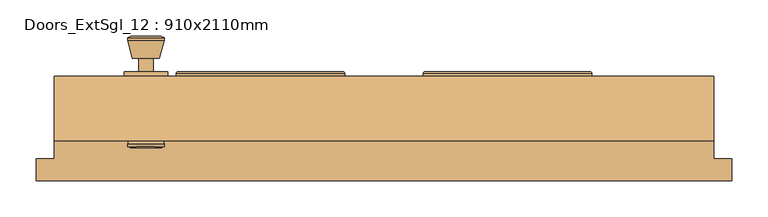
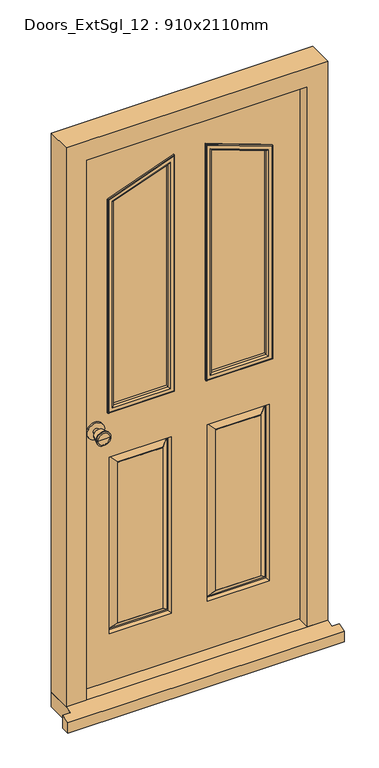
"""IFC4 building model written with IfcOpenShell, lengths in millimetres: door geometry, Doors_ExtSgl_12 : 910x2110mm."""

from ifc_helpers import new_model, si_unit, point, frame, frame_2d, origin, place, context, project, spatial, polyline, circle_curve, ellipse_curve, trimmed, segment, composite_curve, outline, extrude, faceted_brep, source, transform, mapped, element, save
from ifc_brep_helpers import plane_surface, cylinder_surface, revolved_surface, advanced_brep


def doors_extsgl_12_910x2110mm_ece77ece(model_context):
    return source(origin(), model_context, "Body", "SolidModel", [
        advanced_brep(
        [(-328.5, 18.4, 1000.0), (-338.5, 18.4, 1000.0), (-318.5, 18.4, 1000.0), (-308.0241324, 67.4, 1000.0), (-348.9758676, 67.4, 1000.0), (-328.5, 67.4, 1000.0), (-303.5, 65.5721319, 1000.0), (-353.5, 65.5721319, 1000.0), (-303.5, 62.1084537, 1000.0), (-353.5, 62.1084537, 1000.0), (-309.863764, 37.4, 1000.0), (-347.136236, 37.4, 1000.0), (-318.5, 37.4, 1000.0), (-338.5, 37.4, 1000.0)],
        [
            (0, 1),
            (1, 2, circle_curve(frame((-328.5, 18.4, 1000.0), z_axis=(0.0, -1.0, 0.0), x_axis=(-1.0, 0.0, 0.0)), 10.0)),
            (2, 0),
            (2, 1, circle_curve(frame((-328.5, 18.4, 1000.0), z_axis=(0.0, -1.0, 0.0), x_axis=(-1.0, 0.0, 0.0)), 10.0)),
            (3, 4, circle_curve(frame((-328.5, 67.4, 1000.0), z_axis=(0.0, 1.0, 0.0), x_axis=(-1.0, 0.0, 0.0)), 20.4758676)),
            (4, 5),
            (5, 3),
            (4, 3, circle_curve(frame((-328.5, 67.4, 1000.0), z_axis=(0.0, 1.0, 0.0), x_axis=(-1.0, 0.0, 0.0)), 20.4758676)),
            (6, 7, circle_curve(frame((-328.5, 65.5721319, 1000.0), z_axis=(0.0, 1.0, 0.0), x_axis=(-1.0, 0.0, 0.0)), 25.0)),
            (7, 4),
            (3, 6),
            (7, 6, circle_curve(frame((-328.5, 65.5721319, 1000.0), z_axis=(0.0, 1.0, 0.0), x_axis=(-1.0, 0.0, 0.0)), 25.0)),
            (8, 9, circle_curve(frame((-328.5, 62.1084537, 1000.0), z_axis=(0.0, 1.0, 0.0), x_axis=(-1.0, 0.0, 0.0)), 25.0)),
            (9, 7),
            (6, 8),
            (9, 8, circle_curve(frame((-328.5, 62.1084537, 1000.0), z_axis=(0.0, 1.0, 0.0), x_axis=(-1.0, 0.0, 0.0)), 25.0)),
            (10, 11, circle_curve(frame((-328.5, 37.4, 1000.0), z_axis=(0.0, 1.0, 0.0), x_axis=(-1.0, 0.0, 0.0)), 18.636236)),
            (11, 9),
            (8, 10),
            (11, 10, circle_curve(frame((-328.5, 37.4, 1000.0), z_axis=(0.0, 1.0, 0.0), x_axis=(-1.0, 0.0, 0.0)), 18.636236)),
            (12, 13, circle_curve(frame((-328.5, 37.4, 1000.0), z_axis=(0.0, 1.0, 0.0), x_axis=(-1.0, 0.0, 0.0)), 10.0)),
            (13, 11),
            (10, 12),
            (13, 12, circle_curve(frame((-328.5, 37.4, 1000.0), z_axis=(0.0, 1.0, 0.0), x_axis=(-1.0, 0.0, 0.0)), 10.0)),
            (1, 13),
            (12, 2),
        ],
        [
            plane_surface(frame((-328.5, 18.4, 1000.0), z_axis=(0.0, -1.0, 0.0), x_axis=(-1.0, 0.0, 0.0))),
            plane_surface(frame((-328.5, 67.4, 1000.0), z_axis=(0.0, 1.0, 0.0), x_axis=(-1.0, 0.0, 0.0))),
            revolved_surface(polyline([(-348.9758676, 67.4, 1000.0), (-353.5, 65.5721319, 1000.0)]), (-328.5, 18.4, 1000.0), (0.0, -1.0, 0.0)),
            cylinder_surface(frame((-328.5, 18.4, 1000.0), z_axis=(0.0, -1.0, 0.0), x_axis=(-1.0, 0.0, 0.0)), 25.0),
            revolved_surface(polyline([(-353.5, 62.1084537, 1000.0), (-347.136236, 37.4, 1000.0)]), (-328.5, 18.4, 1000.0), (0.0, -1.0, 0.0)),
            plane_surface(frame((-328.5, 37.4, 1000.0), z_axis=(0.0, -1.0, 0.0), x_axis=(-1.0, 0.0, 0.0))),
            cylinder_surface(frame((-328.5, 18.4, 1000.0), z_axis=(0.0, -1.0, 0.0), x_axis=(-1.0, 0.0, 0.0)), 10.0),
        ],
        [
            (0, [[1, 2, 3]]),
            (0, [[-3, 4, -1]]),
            (1, [[5, 6, 7]]),
            (1, [[8, -7, -6]]),
            (2, [[9, 10, -5, 11]]),
            (2, [[12, -11, -8, -10]]),
            (3, [[13, 14, -9, 15]]),
            (3, [[16, -15, -12, -14]]),
            (4, [[17, 18, -13, 19]]),
            (4, [[20, -19, -16, -18]]),
            (5, [[21, 22, -17, 23]]),
            (5, [[24, -23, -20, -22]]),
            (6, [[-2, 25, -21, 26]]),
            (6, [[-4, -26, -24, -25]]),
        ],
    ),
        extrude(outline(composite_curve([segment(trimmed(circle_curve(frame_2d((1000.0, -328.5)), 30.0), [point((1000.0, -358.5))], [point((1000.0, -298.5))], False, "CARTESIAN"), True, "CONTINUOUS"), segment(trimmed(circle_curve(frame_2d((1000.0, -328.5)), 30.0), [point((1000.0, -298.5))], [point((1000.0, -358.5))], False, "CARTESIAN"), True, "CONTINUOUS")], self_intersect=False)), frame((0.0, 12.4, 0.0), z_axis=(0.0, 1.0, 0.0), x_axis=(0.0, 0.0, 1.0)), (0.0, 0.0, 1.0), 6.0),
        advanced_brep(
        [(-328.5, -37.6, 1000.0), (-318.5, -37.6, 1000.0), (-338.5, -37.6, 1000.0), (-308.0241324, -86.6, 1000.0), (-328.5, -86.6, 1000.0), (-348.9758676, -86.6, 1000.0), (-303.5, -84.7721319, 1000.0), (-353.5, -84.7721319, 1000.0), (-303.5, -81.3084537, 1000.0), (-353.5, -81.3084537, 1000.0), (-309.863764, -56.6, 1000.0), (-347.136236, -56.6, 1000.0), (-318.5, -56.6, 1000.0), (-338.5, -56.6, 1000.0)],
        [
            (0, 1),
            (1, 2, circle_curve(frame((-328.5, -37.6, 1000.0), z_axis=(0.0, 1.0, 0.0), x_axis=(-1.0, 0.0, 0.0)), 10.0)),
            (2, 0),
            (2, 1, circle_curve(frame((-328.5, -37.6, 1000.0), z_axis=(0.0, 1.0, 0.0), x_axis=(-1.0, 0.0, 0.0)), 10.0)),
            (3, 4),
            (4, 5),
            (5, 3, circle_curve(frame((-328.5, -86.6, 1000.0), z_axis=(0.0, -1.0, 0.0), x_axis=(-1.0, 0.0, 0.0)), 20.4758676)),
            (3, 5, circle_curve(frame((-328.5, -86.6, 1000.0), z_axis=(0.0, -1.0, 0.0), x_axis=(-1.0, 0.0, 0.0)), 20.4758676)),
            (6, 3),
            (5, 7),
            (7, 6, circle_curve(frame((-328.5, -84.7721319, 1000.0), z_axis=(0.0, -1.0, 0.0), x_axis=(-1.0, 0.0, 0.0)), 25.0)),
            (6, 7, circle_curve(frame((-328.5, -84.7721319, 1000.0), z_axis=(0.0, -1.0, 0.0), x_axis=(-1.0, 0.0, 0.0)), 25.0)),
            (8, 6),
            (7, 9),
            (9, 8, circle_curve(frame((-328.5, -81.3084537, 1000.0), z_axis=(0.0, -1.0, 0.0), x_axis=(-1.0, 0.0, 0.0)), 25.0)),
            (8, 9, circle_curve(frame((-328.5, -81.3084537, 1000.0), z_axis=(0.0, -1.0, 0.0), x_axis=(-1.0, 0.0, 0.0)), 25.0)),
            (10, 8),
            (9, 11),
            (11, 10, circle_curve(frame((-328.5, -56.6, 1000.0), z_axis=(0.0, -1.0, 0.0), x_axis=(-1.0, 0.0, 0.0)), 18.636236)),
            (10, 11, circle_curve(frame((-328.5, -56.6, 1000.0), z_axis=(0.0, -1.0, 0.0), x_axis=(-1.0, 0.0, 0.0)), 18.636236)),
            (12, 10),
            (11, 13),
            (13, 12, circle_curve(frame((-328.5, -56.6, 1000.0), z_axis=(0.0, -1.0, 0.0), x_axis=(-1.0, 0.0, 0.0)), 10.0)),
            (12, 13, circle_curve(frame((-328.5, -56.6, 1000.0), z_axis=(0.0, -1.0, 0.0), x_axis=(-1.0, 0.0, 0.0)), 10.0)),
            (1, 12),
            (13, 2),
        ],
        [
            plane_surface(frame((-328.5, -37.6, 1000.0), z_axis=(0.0, 1.0, 0.0), x_axis=(-1.0, 0.0, 0.0))),
            plane_surface(frame((-328.5, -86.6, 1000.0), z_axis=(0.0, -1.0, 0.0), x_axis=(-1.0, 0.0, 0.0))),
            revolved_surface(polyline([(-348.9758676, -86.6, 1000.0), (-353.5, -84.7721319, 1000.0)]), (-328.5, -37.6, 1000.0), (0.0, 1.0, 0.0)),
            cylinder_surface(frame((-328.5, -37.6, 1000.0), z_axis=(0.0, 1.0, 0.0), x_axis=(-1.0, 0.0, 0.0)), 25.0),
            revolved_surface(polyline([(-353.5, -81.3084537, 1000.0), (-347.136236, -56.6, 1000.0)]), (-328.5, -37.6, 1000.0), (0.0, 1.0, 0.0)),
            plane_surface(frame((-328.5, -56.6, 1000.0), z_axis=(0.0, 1.0, 0.0), x_axis=(-1.0, 0.0, 0.0))),
            cylinder_surface(frame((-328.5, -37.6, 1000.0), z_axis=(0.0, 1.0, 0.0), x_axis=(-1.0, 0.0, 0.0)), 10.0),
        ],
        [
            (0, [[1, 2, 3]]),
            (0, [[-3, 4, -1]]),
            (1, [[5, 6, 7]]),
            (1, [[-6, -5, 8]]),
            (2, [[9, -7, 10, 11]]),
            (2, [[-10, -8, -9, 12]]),
            (3, [[13, -11, 14, 15]]),
            (3, [[-14, -12, -13, 16]]),
            (4, [[17, -15, 18, 19]]),
            (4, [[-18, -16, -17, 20]]),
            (5, [[21, -19, 22, 23]]),
            (5, [[-22, -20, -21, 24]]),
            (6, [[25, -23, 26, -2]]),
            (6, [[-26, -24, -25, -4]]),
        ],
    ),
        extrude(outline(composite_curve([segment(trimmed(circle_curve(frame_2d((1000.0, -328.5)), 30.0), [point((1000.0, -358.5))], [point((1000.0, -298.5))], False, "CARTESIAN"), True, "CONTINUOUS"), segment(trimmed(circle_curve(frame_2d((1000.0, -328.5)), 30.0), [point((1000.0, -298.5))], [point((1000.0, -358.5))], False, "CARTESIAN"), True, "CONTINUOUS")], self_intersect=False)), frame((0.0, -37.6, 0.0), z_axis=(0.0, 1.0, 0.0), x_axis=(0.0, 0.0, 1.0)), (0.0, 0.0, 1.0), 6.0),
        faceted_brep([(384.5, -76.6, 54.5), (384.5, -34.6, 54.5), (406.5, -34.6, 54.5), (406.5, 12.4, 54.5), (455.0, 12.4, 54.5), (455.0, -76.6, 54.5), (455.0, -76.6, 2110.0), (-455.0, -76.6, 2110.0), (-455.0, -76.6, 54.5), (-384.5, -76.6, 54.5), (-384.5, -76.6, 2039.5), (384.5, -76.6, 2039.5), (455.0, 12.4, 2110.0), (406.5, 12.4, 2061.5), (-406.5, 12.4, 2061.5), (-406.5, 12.4, 54.5), (-455.0, 12.4, 54.5), (-455.0, 12.4, 2110.0), (406.5, -34.6, 2061.5), (384.5, -34.6, 2039.5), (-384.5, -34.6, 2039.5), (-384.5, -34.6, 54.5), (-406.5, -34.6, 54.5), (-406.5, -34.6, 2061.5)], [[[0, 1, 2, 3, 4, 5]], [[5, 6, 7, 8, 9, 10, 11, 0]], [[4, 12, 6, 5]], [[3, 13, 14, 15, 16, 17, 12, 4]], [[2, 18, 13, 3]], [[1, 19, 20, 21, 22, 23, 18, 2]], [[0, 11, 19, 1]], [[9, 21, 20, 10]], [[8, 16, 15, 22, 21, 9]], [[7, 17, 16, 8]], [[14, 23, 22, 15]], [[6, 12, 17, 7]], [[13, 18, 23, 14]], [[10, 20, 19, 11]]]),
        faceted_brep([(403.5, 12.4, 58.5), (-404.4250294, 12.4, 58.5), (-404.4250294, 12.4, 2058.5), (403.5, 12.4, 2058.5), (62.5, 12.4, 1058.5), (278.5, 12.4, 1058.5), (278.5, 12.4, 1829.8824294), (62.5, 12.4, 1908.5), (-278.5, 12.4, 1058.5), (-62.5, 12.4, 1058.5), (-62.5, 12.4, 1908.5), (-278.5, 12.4, 1829.8824294), (-62.5, 12.4, 883.5), (-278.5, 12.4, 883.5), (-278.5, 12.4, 233.5), (-62.5, 12.4, 233.5), (278.5, 12.4, 883.5), (62.5, 12.4, 883.5), (62.5, 12.4, 233.5), (278.5, 12.4, 233.5), (-92.5, 12.4, 263.5), (-248.5, 12.4, 263.5), (-248.5, 12.4, 853.5), (-92.5, 12.4, 853.5), (248.5, 12.4, 263.5), (92.5, 12.4, 263.5), (92.5, 12.4, 853.5), (248.5, 12.4, 853.5), (403.5, -31.6, 58.5), (403.5, -31.6, 2058.5), (-404.4250294, -31.6, 2058.5), (-404.4250294, -31.6, 58.5), (62.5, -31.6, 1058.5), (62.5, -31.6, 1908.5), (278.5, -31.6, 1829.8824294), (278.5, -31.6, 1058.5), (-278.5, -31.6, 1058.5), (-278.5, -31.6, 1829.8824294), (-62.5, -31.6, 1908.5), (-62.5, -31.6, 1058.5), (62.5, -31.6, 883.5), (278.5, -31.6, 883.5), (278.5, -31.6, 233.5), (62.5, -31.6, 233.5), (-278.5, -31.6, 883.5), (-62.5, -31.6, 883.5), (-62.5, -31.6, 233.5), (-278.5, -31.6, 233.5), (92.5, -31.6, 263.5), (248.5, -31.6, 263.5), (248.5, -31.6, 853.5), (92.5, -31.6, 853.5), (-248.5, -31.6, 263.5), (-92.5, -31.6, 263.5), (-92.5, -31.6, 853.5), (-248.5, -31.6, 853.5), (65.5, -16.6, 880.5), (65.5, -16.6, 236.5), (90.5, -30.6, 855.5), (70.5, -16.6, 875.5), (70.5, -16.6, 241.5), (90.5, -30.6, 261.5), (92.5, -30.6, 853.5), (92.5, -30.6, 263.5), (275.5, -16.6, 236.5), (270.5, -16.6, 241.5), (250.5, -30.6, 261.5), (248.5, -30.6, 263.5), (275.5, -16.6, 880.5), (270.5, -16.6, 875.5), (250.5, -30.6, 855.5), (248.5, -30.6, 853.5), (-275.5, -16.6, 880.5), (-275.5, -16.6, 236.5), (-250.5, -30.6, 855.5), (-270.5, -16.6, 875.5), (-270.5, -16.6, 241.5), (-250.5, -30.6, 261.5), (-248.5, -30.6, 853.5), (-248.5, -30.6, 263.5), (-65.5, -16.6, 236.5), (-70.5, -16.6, 241.5), (-90.5, -30.6, 261.5), (-92.5, -30.6, 263.5), (-65.5, -16.6, 880.5), (-70.5, -16.6, 875.5), (-90.5, -30.6, 855.5), (-92.5, -30.6, 853.5), (-92.5, 11.4, 263.5), (-92.5, 11.4, 853.5), (-70.5, -2.6, 241.5), (-90.5, 11.4, 261.5), (-90.5, 11.4, 855.5), (-70.5, -2.6, 875.5), (-65.5, -2.6, 236.5), (-65.5, -2.6, 880.5), (-248.5, 11.4, 853.5), (-250.5, 11.4, 855.5), (-270.5, -2.6, 875.5), (-275.5, -2.6, 880.5), (-248.5, 11.4, 263.5), (-250.5, 11.4, 261.5), (-270.5, -2.6, 241.5), (-275.5, -2.6, 236.5), (275.5, -2.6, 880.5), (275.5, -2.6, 236.5), (250.5, 11.4, 855.5), (270.5, -2.6, 875.5), (270.5, -2.6, 241.5), (250.5, 11.4, 261.5), (248.5, 11.4, 853.5), (248.5, 11.4, 263.5), (65.5, -2.6, 236.5), (70.5, -2.6, 241.5), (90.5, 11.4, 261.5), (92.5, 11.4, 263.5), (65.5, -2.6, 880.5), (70.5, -2.6, 875.5), (90.5, 11.4, 855.5), (92.5, 11.4, 853.5)], [[[0, 1, 2, 3], [4, 5, 6, 7], [8, 9, 10, 11], [12, 13, 14, 15], [16, 17, 18, 19]], [[20, 21, 22, 23]], [[24, 25, 26, 27]], [[28, 29, 30, 31], [32, 33, 34, 35], [36, 37, 38, 39], [40, 41, 42, 43], [44, 45, 46, 47]], [[48, 49, 50, 51]], [[52, 53, 54, 55]], [[3, 29, 28, 0]], [[2, 30, 29, 3]], [[1, 31, 30, 2]], [[0, 28, 31, 1]], [[7, 33, 32, 4]], [[6, 34, 33, 7]], [[5, 35, 34, 6]], [[4, 32, 35, 5]], [[11, 37, 36, 8]], [[10, 38, 37, 11]], [[9, 39, 38, 10]], [[8, 36, 39, 9]], [[56, 40, 43, 57]], [[58, 59, 60, 61]], [[48, 51, 62, 63]], [[43, 42, 64, 57]], [[60, 65, 66, 61]], [[63, 67, 49, 48]], [[42, 41, 68, 64]], [[65, 69, 70, 66]], [[67, 71, 50, 49]], [[56, 68, 41, 40]], [[57, 64, 68, 56], [59, 69, 65, 60]], [[58, 70, 69, 59]], [[61, 66, 70, 58], [62, 71, 67, 63]], [[51, 50, 71, 62]], [[72, 44, 47, 73]], [[74, 75, 76, 77]], [[52, 55, 78, 79]], [[47, 46, 80, 73]], [[76, 81, 82, 77]], [[79, 83, 53, 52]], [[46, 45, 84, 80]], [[81, 85, 86, 82]], [[83, 87, 54, 53]], [[72, 84, 45, 44]], [[73, 80, 84, 72], [75, 85, 81, 76]], [[74, 86, 85, 75]], [[77, 82, 86, 74], [78, 87, 83, 79]], [[55, 54, 87, 78]], [[88, 20, 23, 89]], [[90, 91, 92, 93]], [[12, 15, 94, 95]], [[23, 22, 96, 89]], [[92, 97, 98, 93]], [[95, 99, 13, 12]], [[22, 21, 100, 96]], [[97, 101, 102, 98]], [[99, 103, 14, 13]], [[88, 100, 21, 20]], [[91, 101, 97, 92], [89, 96, 100, 88]], [[90, 102, 101, 91]], [[94, 103, 99, 95], [93, 98, 102, 90]], [[15, 14, 103, 94]], [[104, 16, 19, 105]], [[106, 107, 108, 109]], [[24, 27, 110, 111]], [[19, 18, 112, 105]], [[108, 113, 114, 109]], [[111, 115, 25, 24]], [[18, 17, 116, 112]], [[113, 117, 118, 114]], [[115, 119, 26, 25]], [[104, 116, 17, 16]], [[105, 112, 116, 104], [107, 117, 113, 108]], [[106, 118, 117, 107]], [[109, 114, 118, 106], [110, 119, 115, 111]], [[27, 26, 119, 110]]]),
        faceted_brep([(480.0, -131.6, 0.0), (480.0, -101.6, 0.0), (480.0, -101.6, 47.2703282), (480.0, -131.6, 38.5947221), (-480.0, -131.6, 38.5947221), (-480.0, -101.6, 47.2703282), (-480.0, -101.6, 0.0), (-480.0, -131.6, 0.0), (-455.0, -101.6, 0.0), (-455.0, 12.4, 0.0), (455.0, 12.4, 0.0), (455.0, -101.6, 0.0), (455.0, -101.6, 47.2703282), (455.0, -76.6, 54.5), (-455.0, -76.6, 54.5), (-455.0, -101.6, 47.2703282), (455.0, 12.4, 54.5), (-455.0, 12.4, 54.5)], [[[0, 1, 2, 3]], [[4, 5, 6, 7]], [[7, 6, 8, 9, 10, 11, 1, 0]], [[3, 4, 7, 0]], [[3, 2, 12, 13, 14, 15, 5, 4]], [[14, 13, 16, 17]], [[17, 16, 10, 9]], [[15, 14, 17, 9, 8]], [[8, 6, 5, 15]], [[11, 10, 16, 13, 12]], [[12, 2, 1, 11]]]),
        extrude(outline(polyline([(1058.5, 278.5), (1829.8824294, 278.5), (1908.5, 62.5), (1058.5, 62.5), (1058.5, 278.5)])), frame((0.0, -21.6, 0.0), z_axis=(0.0, 1.0, 0.0), x_axis=(0.0, 0.0, 1.0)), (0.0, 0.0, 1.0), 24.0),
        extrude(outline(polyline([(1058.5, -62.5), (1908.5, -62.5), (1829.8824294, -278.5), (1058.5, -278.5), (1058.5, -62.5)])), frame((0.0, -21.6, 0.0), z_axis=(0.0, 1.0, 0.0), x_axis=(0.0, 0.0, 1.0)), (0.0, 0.0, 1.0), 24.0),
        advanced_brep(
        [(286.5, -35.6, 1835.4840897), (286.5, -35.6, 1050.5), (286.5, -31.6, 1050.5), (286.5, -31.6, 1835.4840897), (284.5, -37.6, 1834.0836746), (284.5, -37.6, 1052.5), (266.5, -32.6, 1821.4799389), (266.5, -32.6, 1070.5), (271.5, -37.6, 1065.5), (271.5, -37.6, 1824.9809766), (266.5, -21.6, 1821.4799389), (266.5, -21.6, 1070.5), (278.5, -31.6, 1829.8824294), (278.5, -31.6, 1058.5), (278.5, -21.6, 1058.5), (278.5, -21.6, 1829.8824294), (54.5, -35.6, 1050.5), (54.5, -31.6, 1050.5), (56.5, -37.6, 1052.5), (74.5, -32.6, 1070.5), (69.5, -37.6, 1065.5), (74.5, -21.6, 1070.5), (62.5, -31.6, 1058.5), (62.5, -21.6, 1058.5), (54.5, -35.6, 1919.9251841), (54.5, -31.6, 1919.9251841), (56.5, -37.6, 1917.068888), (74.5, -32.6, 1891.3622239), (69.5, -37.6, 1898.502964), (74.5, -21.6, 1891.3622239), (62.5, -31.6, 1908.5), (62.5, -21.6, 1908.5)],
        [
            (0, 1),
            (1, 2),
            (2, 3),
            (3, 0),
            (4, 5),
            (5, 1, ellipse_curve(frame((284.5, -35.6, 1052.5), z_axis=(0.7071067811865475, 0.0, 0.7071067811865475), x_axis=(-0.7071067811865474, 0.0, 0.7071067811865476)), 2.8284271, 2.0)),
            (0, 4, ellipse_curve(frame((284.5, -35.6, 1834.0836746), z_axis=(0.5735764363510463, 0.0, -0.8191520442889918), x_axis=(0.8191520442889918, 0.0, 0.5735764363510459)), 2.4415492, 2.0)),
            (6, 7),
            (7, 8, ellipse_curve(frame((271.5, -32.6, 1065.5), z_axis=(0.7071067811865475, 0.0, 0.7071067811865475), x_axis=(-0.7071067811865474, 0.0, 0.7071067811865476)), 7.0710678, 5.0)),
            (8, 9),
            (9, 6, ellipse_curve(frame((271.5, -32.6, 1824.9809766), z_axis=(0.5735764363510463, 0.0, -0.8191520442889918), x_axis=(0.8191520442889918, 0.0, 0.5735764363510459)), 6.1038729, 5.0)),
            (10, 11),
            (11, 7),
            (6, 10),
            (12, 13),
            (13, 14),
            (14, 15),
            (15, 12),
            (1, 16),
            (16, 17),
            (17, 2),
            (5, 18),
            (18, 16, ellipse_curve(frame((56.5, -35.6, 1052.5), z_axis=(0.7071067811865475, 0.0, -0.7071067811865475), x_axis=(0.7071067811865476, 0.0, 0.7071067811865474)), 2.8284271, 2.0)),
            (7, 19),
            (19, 20, ellipse_curve(frame((69.5, -32.6, 1065.5), z_axis=(0.7071067811865475, 0.0, -0.7071067811865475), x_axis=(0.7071067811865476, 0.0, 0.7071067811865474)), 7.0710678, 5.0)),
            (20, 8),
            (11, 21),
            (21, 19),
            (13, 22),
            (22, 23),
            (23, 14),
            (16, 24),
            (24, 25),
            (25, 17),
            (18, 26),
            (26, 24, ellipse_curve(frame((56.5, -35.6, 1917.068888), z_axis=(-0.8191520442889917, 0.0, -0.5735764363510462), x_axis=(0.5735764363510462, 0.0, -0.8191520442889918)), 3.4868936, 2.0)),
            (19, 27),
            (27, 28, ellipse_curve(frame((69.5, -32.6, 1898.502964), z_axis=(-0.8191520442889917, 0.0, -0.5735764363510462), x_axis=(0.5735764363510462, 0.0, -0.8191520442889918)), 8.717234, 5.0)),
            (28, 20),
            (21, 29),
            (29, 27),
            (22, 30),
            (30, 31),
            (31, 23),
            (24, 0),
            (3, 25),
            (26, 4),
            (28, 9),
            (27, 6),
            (29, 10),
            (31, 15),
            (30, 12),
        ],
        [
            plane_surface(frame((286.5, -31.6, 1835.4840897), z_axis=(1.0, 0.0, 0.0), x_axis=(0.0, 0.0, -1.0))),
            cylinder_surface(frame((284.5, -35.6, 1829.8824294), z_axis=(0.0, 0.0, 1.0), x_axis=(1.0, 0.0, 0.0)), 2.0),
            cylinder_surface(frame((271.5, -32.6, 1829.8824294), z_axis=(0.0, 0.0, 1.0), x_axis=(1.0, 0.0, 0.0)), 5.0),
            plane_surface(frame((266.5, -32.6, 1821.4799389), z_axis=(-1.0, 0.0, 0.0), x_axis=(0.0, 0.0, -1.0))),
            plane_surface(frame((278.5, -21.6, 1829.8824294), z_axis=(1.0, 0.0, 0.0), x_axis=(0.0, 0.0, -1.0))),
            plane_surface(frame((286.5, -31.6, 1050.5), z_axis=(0.0, 0.0, -1.0), x_axis=(-1.0, 0.0, 0.0))),
            cylinder_surface(frame((278.5, -35.6, 1052.5), z_axis=(1.0, 0.0, 0.0), x_axis=(0.0, 0.0, -1.0)), 2.0),
            cylinder_surface(frame((278.5, -32.6, 1065.5), z_axis=(1.0, 0.0, 0.0), x_axis=(0.0, 0.0, -1.0)), 5.0),
            plane_surface(frame((266.5, -32.6, 1070.5), z_axis=(0.0, 0.0, 1.0), x_axis=(-1.0, 0.0, 0.0))),
            plane_surface(frame((278.5, -21.6, 1058.5), z_axis=(0.0, 0.0, -1.0), x_axis=(-1.0, 0.0, 0.0))),
            plane_surface(frame((54.5, -31.6, 1050.5), z_axis=(-1.0, 0.0, 0.0), x_axis=(0.0, 0.0, 1.0))),
            cylinder_surface(frame((56.5, -35.6, 1058.5), z_axis=(0.0, 0.0, -1.0), x_axis=(-1.0, 0.0, 0.0)), 2.0),
            cylinder_surface(frame((69.5, -32.6, 1058.5), z_axis=(0.0, 0.0, -1.0), x_axis=(-1.0, 0.0, 0.0)), 5.0),
            plane_surface(frame((74.5, -32.6, 1070.5), z_axis=(1.0, 0.0, 0.0), x_axis=(0.0, 0.0, 1.0))),
            plane_surface(frame((62.5, -21.6, 1058.5), z_axis=(-1.0, 0.0, 0.0), x_axis=(0.0, 0.0, 1.0))),
            plane_surface(frame((54.5, -31.6, 1919.9251841), z_axis=(0.3420201433256683, 0.0, 0.9396926207859085), x_axis=(0.9396926207859085, 0.0, -0.3420201433256683))),
            cylinder_surface(frame((64.5521209, -35.6, 1914.1381557), z_axis=(-0.9396926207859085, 0.0, 0.34202014332566844), x_axis=(0.34202014332566844, 0.0, 0.9396926207859085)), 2.0),
            plane_surface(frame((56.5, -37.6, 1917.068888), z_axis=(0.0, -1.0, 0.0), x_axis=(0.9396926207859085, 0.0, -0.34202014332566844))),
            cylinder_surface(frame((60.105859, -32.6, 1901.9221517), z_axis=(-0.9396926207859085, 0.0, 0.34202014332566844), x_axis=(0.34202014332566844, 0.0, 0.9396926207859085)), 5.0),
            plane_surface(frame((74.5, -32.6, 1891.3622239), z_axis=(-0.34202014332566844, 0.0, -0.9396926207859085), x_axis=(0.9396926207859085, 0.0, -0.34202014332566844))),
            plane_surface(frame((74.5, -21.6, 1891.3622239), z_axis=(0.0, 1.0, 0.0), x_axis=(0.9396926207859088, 0.0, -0.3420201433256677))),
            plane_surface(frame((62.5, -21.6, 1908.5), z_axis=(0.34202014332566905, 0.0, 0.9396926207859083), x_axis=(0.9396926207859083, 0.0, -0.34202014332566905))),
            plane_surface(frame((62.5, -31.6, 1908.5), z_axis=(0.0, 1.0, 0.0), x_axis=(0.9396926207859083, 0.0, -0.3420201433256691))),
        ],
        [
            (0, [[1, 2, 3, 4]]),
            (1, [[5, 6, -1, 7]]),
            (2, [[8, 9, 10, 11]]),
            (3, [[12, 13, -8, 14]]),
            (4, [[15, 16, 17, 18]]),
            (5, [[19, 20, 21, -2]]),
            (6, [[22, 23, -19, -6]]),
            (7, [[24, 25, 26, -9]]),
            (8, [[27, 28, -24, -13]]),
            (9, [[29, 30, 31, -16]]),
            (10, [[32, 33, 34, -20]]),
            (11, [[35, 36, -32, -23]]),
            (12, [[37, 38, 39, -25]]),
            (13, [[40, 41, -37, -28]]),
            (14, [[42, 43, 44, -30]]),
            (15, [[45, -4, 46, -33]]),
            (16, [[47, -7, -45, -36]]),
            (17, [[-5, -47, -35, -22], [-10, -26, -39, 48]]),
            (18, [[49, -11, -48, -38]]),
            (19, [[50, -14, -49, -41]]),
            (20, [[-17, -31, -44, 51], [-12, -50, -40, -27]]),
            (21, [[52, -18, -51, -43]]),
            (22, [[-3, -21, -34, -46], [-15, -52, -42, -29]]),
        ],
    ),
        advanced_brep(
        [(-54.5, -35.6, 1050.5), (-286.5, -35.6, 1050.5), (-286.5, -31.6, 1050.5), (-54.5, -31.6, 1050.5), (-56.5, -37.6, 1052.5), (-284.5, -37.6, 1052.5), (-74.5, -32.6, 1070.5), (-266.5, -32.6, 1070.5), (-271.5, -37.6, 1065.5), (-69.5, -37.6, 1065.5), (-74.5, -21.6, 1070.5), (-266.5, -21.6, 1070.5), (-62.5, -31.6, 1058.5), (-278.5, -31.6, 1058.5), (-278.5, -21.6, 1058.5), (-62.5, -21.6, 1058.5), (-286.5, -35.6, 1835.4840897), (-286.5, -31.6, 1835.4840897), (-284.5, -37.6, 1834.0836746), (-266.5, -32.6, 1821.4799389), (-271.5, -37.6, 1824.9809766), (-266.5, -21.6, 1821.4799389), (-278.5, -31.6, 1829.8824294), (-278.5, -21.6, 1829.8824294), (-54.5, -35.6, 1919.9251841), (-54.5, -31.6, 1919.9251841), (-56.5, -37.6, 1917.068888), (-74.5, -32.6, 1891.3622239), (-69.5, -37.6, 1898.502964), (-74.5, -21.6, 1891.3622239), (-62.5, -31.6, 1908.5), (-62.5, -21.6, 1908.5)],
        [
            (0, 1),
            (1, 2),
            (2, 3),
            (3, 0),
            (4, 5),
            (5, 1, ellipse_curve(frame((-284.5, -35.6, 1052.5), z_axis=(0.7071067811865476, 0.0, -0.7071067811865475), x_axis=(0.7071067811865475, 0.0, 0.7071067811865475)), 2.8284271, 2.0)),
            (0, 4, ellipse_curve(frame((-56.5, -35.6, 1052.5), z_axis=(-0.7071067811865475, 0.0, -0.7071067811865475), x_axis=(0.7071067811865476, 0.0, -0.7071067811865475)), 2.8284271, 2.0)),
            (6, 7),
            (7, 8, ellipse_curve(frame((-271.5, -32.6, 1065.5), z_axis=(0.7071067811865476, 0.0, -0.7071067811865475), x_axis=(0.7071067811865475, 0.0, 0.7071067811865475)), 7.0710678, 5.0)),
            (8, 9),
            (9, 6, ellipse_curve(frame((-69.5, -32.6, 1065.5), z_axis=(-0.7071067811865475, 0.0, -0.7071067811865475), x_axis=(0.7071067811865476, 0.0, -0.7071067811865475)), 7.0710678, 5.0)),
            (10, 11),
            (11, 7),
            (6, 10),
            (12, 13),
            (13, 14),
            (14, 15),
            (15, 12),
            (1, 16),
            (16, 17),
            (17, 2),
            (5, 18),
            (18, 16, ellipse_curve(frame((-284.5, -35.6, 1834.0836746), z_axis=(-0.5735764363510245, 0.0, -0.8191520442890069), x_axis=(0.8191520442890068, 0.0, -0.5735764363510246)), 2.4415492, 2.0)),
            (7, 19),
            (19, 20, ellipse_curve(frame((-271.5, -32.6, 1824.9809766), z_axis=(-0.5735764363510245, 0.0, -0.8191520442890069), x_axis=(0.8191520442890068, 0.0, -0.5735764363510246)), 6.1038729, 5.0)),
            (20, 8),
            (11, 21),
            (21, 19),
            (13, 22),
            (22, 23),
            (23, 14),
            (16, 24),
            (24, 25),
            (25, 17),
            (18, 26),
            (26, 24, ellipse_curve(frame((-56.5, -35.6, 1917.068888), z_axis=(-0.8191520442890069, 0.0, 0.5735764363510246), x_axis=(-0.5735764363510246, 0.0, -0.8191520442890069)), 3.4868936, 2.0)),
            (19, 27),
            (27, 28, ellipse_curve(frame((-69.5, -32.6, 1898.502964), z_axis=(-0.8191520442890069, 0.0, 0.5735764363510246), x_axis=(-0.5735764363510246, 0.0, -0.8191520442890069)), 8.717234, 5.0)),
            (28, 20),
            (21, 29),
            (29, 27),
            (22, 30),
            (30, 31),
            (31, 23),
            (24, 0),
            (3, 25),
            (26, 4),
            (28, 9),
            (27, 6),
            (29, 10),
            (31, 15),
            (30, 12),
        ],
        [
            plane_surface(frame((-54.5, -31.6, 1050.5), z_axis=(0.0, 0.0, -1.0), x_axis=(-1.0, 0.0, 0.0))),
            cylinder_surface(frame((-62.5, -35.6, 1052.5), z_axis=(1.0, 0.0, 0.0), x_axis=(0.0, 0.0, -1.0)), 2.0),
            cylinder_surface(frame((-62.5, -32.6, 1065.5), z_axis=(1.0, 0.0, 0.0), x_axis=(0.0, 0.0, -1.0)), 5.0),
            plane_surface(frame((-74.5, -32.6, 1070.5), z_axis=(0.0, 0.0, 1.0), x_axis=(-1.0, 0.0, 0.0))),
            plane_surface(frame((-62.5, -21.6, 1058.5), z_axis=(0.0, 0.0, -1.0), x_axis=(-1.0, 0.0, 0.0))),
            plane_surface(frame((-286.5, -31.6, 1050.5), z_axis=(-1.0, 0.0, 0.0), x_axis=(0.0, 0.0, 1.0))),
            cylinder_surface(frame((-284.5, -35.6, 1058.5), z_axis=(0.0, 0.0, -1.0), x_axis=(-1.0, 0.0, 0.0)), 2.0),
            cylinder_surface(frame((-271.5, -32.6, 1058.5), z_axis=(0.0, 0.0, -1.0), x_axis=(-1.0, 0.0, 0.0)), 5.0),
            plane_surface(frame((-266.5, -32.6, 1070.5), z_axis=(1.0, 0.0, 0.0), x_axis=(0.0, 0.0, 1.0))),
            plane_surface(frame((-278.5, -21.6, 1058.5), z_axis=(-1.0, 0.0, 0.0), x_axis=(0.0, 0.0, 1.0))),
            plane_surface(frame((-286.5, -31.6, 1835.4840897), z_axis=(-0.34202014332571895, 0.0, 0.9396926207858901), x_axis=(0.9396926207858901, 0.0, 0.34202014332571895))),
            cylinder_surface(frame((-280.5521209, -35.6, 1835.5205851), z_axis=(-0.9396926207858904, 0.0, -0.3420201433257182), x_axis=(-0.3420201433257182, 0.0, 0.9396926207858904)), 2.0),
            cylinder_surface(frame((-276.105859, -32.6, 1823.3045811), z_axis=(-0.9396926207858904, 0.0, -0.3420201433257182), x_axis=(-0.3420201433257182, 0.0, 0.9396926207858904)), 5.0),
            plane_surface(frame((-266.5, -32.6, 1821.4799389), z_axis=(0.3420201433257189, 0.0, -0.9396926207858901), x_axis=(0.9396926207858901, 0.0, 0.3420201433257189))),
            plane_surface(frame((-278.5, -21.6, 1829.8824294), z_axis=(-0.3420201433257181, 0.0, 0.9396926207858906), x_axis=(0.9396926207858906, 0.0, 0.3420201433257181))),
            plane_surface(frame((-54.5, -31.6, 1919.9251841), z_axis=(1.0, 0.0, 0.0), x_axis=(0.0, 0.0, -1.0))),
            cylinder_surface(frame((-56.5, -35.6, 1908.5), z_axis=(0.0, 0.0, 1.0), x_axis=(1.0, 0.0, 0.0)), 2.0),
            plane_surface(frame((-56.5, -37.6, 1917.068888), z_axis=(0.0, -1.0, 0.0), x_axis=(0.0, 0.0, -1.0))),
            cylinder_surface(frame((-69.5, -32.6, 1908.5), z_axis=(0.0, 0.0, 1.0), x_axis=(1.0, 0.0, 0.0)), 5.0),
            plane_surface(frame((-74.5, -32.6, 1891.3622239), z_axis=(-1.0, 0.0, 0.0), x_axis=(0.0, 0.0, -1.0))),
            plane_surface(frame((-74.5, -21.6, 1891.3622239), z_axis=(0.0, 1.0, 0.0), x_axis=(0.0, 0.0, -1.0))),
            plane_surface(frame((-62.5, -21.6, 1908.5), z_axis=(1.0, 0.0, 0.0), x_axis=(0.0, 0.0, -1.0))),
            plane_surface(frame((-62.5, -31.6, 1908.5), z_axis=(0.0, 1.0, 0.0), x_axis=(0.0, 0.0, -1.0))),
        ],
        [
            (0, [[1, 2, 3, 4]]),
            (1, [[5, 6, -1, 7]]),
            (2, [[8, 9, 10, 11]]),
            (3, [[12, 13, -8, 14]]),
            (4, [[15, 16, 17, 18]]),
            (5, [[19, 20, 21, -2]]),
            (6, [[22, 23, -19, -6]]),
            (7, [[24, 25, 26, -9]]),
            (8, [[27, 28, -24, -13]]),
            (9, [[29, 30, 31, -16]]),
            (10, [[32, 33, 34, -20]]),
            (11, [[35, 36, -32, -23]]),
            (12, [[37, 38, 39, -25]]),
            (13, [[40, 41, -37, -28]]),
            (14, [[42, 43, 44, -30]]),
            (15, [[45, -4, 46, -33]]),
            (16, [[47, -7, -45, -36]]),
            (17, [[-5, -47, -35, -22], [-10, -26, -39, 48]]),
            (18, [[49, -11, -48, -38]]),
            (19, [[50, -14, -49, -41]]),
            (20, [[-17, -31, -44, 51], [-12, -50, -40, -27]]),
            (21, [[52, -18, -51, -43]]),
            (22, [[-3, -21, -34, -46], [-15, -52, -42, -29]]),
        ],
    ),
        advanced_brep(
        [(-278.5, 2.4, 1829.8824294), (-62.5, 2.4, 1908.5), (-62.5, 12.4, 1908.5), (-278.5, 12.4, 1829.8824294), (-266.5, 13.4, 1821.4799389), (-74.5, 13.4, 1891.3622239), (-74.5, 2.4, 1891.3622239), (-266.5, 2.4, 1821.4799389), (-271.5, 18.4, 1824.9809766), (-69.5, 18.4, 1898.502964), (-286.5, 16.4, 1835.4840897), (-54.5, 16.4, 1919.9251841), (-56.5, 18.4, 1917.068888), (-284.5, 18.4, 1834.0836746), (-286.5, 12.4, 1835.4840897), (-54.5, 12.4, 1919.9251841), (-62.5, 2.4, 1058.5), (-62.5, 12.4, 1058.5), (-74.5, 13.4, 1070.5), (-74.5, 2.4, 1070.5), (-69.5, 18.4, 1065.5), (-54.5, 16.4, 1050.5), (-56.5, 18.4, 1052.5), (-54.5, 12.4, 1050.5), (-278.5, 2.4, 1058.5), (-278.5, 12.4, 1058.5), (-266.5, 13.4, 1070.5), (-266.5, 2.4, 1070.5), (-271.5, 18.4, 1065.5), (-286.5, 16.4, 1050.5), (-284.5, 18.4, 1052.5), (-286.5, 12.4, 1050.5)],
        [
            (0, 1),
            (1, 2),
            (2, 3),
            (3, 0),
            (4, 5),
            (5, 6),
            (6, 7),
            (7, 4),
            (8, 9),
            (9, 5, ellipse_curve(frame((-69.5, 13.4, 1898.502964), z_axis=(-0.8191520442890071, 0.0, 0.5735764363510244), x_axis=(-0.5735764363510243, 0.0, -0.8191520442890072)), 8.717234, 5.0)),
            (4, 8, ellipse_curve(frame((-271.5, 13.4, 1824.9809766), z_axis=(0.5735764363510244, 0.0, 0.819152044289007), x_axis=(-0.8191520442890069, 0.0, 0.5735764363510246)), 6.1038729, 5.0)),
            (10, 11),
            (11, 12, ellipse_curve(frame((-56.5, 16.4, 1917.068888), z_axis=(-0.8191520442890071, 0.0, 0.5735764363510244), x_axis=(-0.5735764363510243, 0.0, -0.8191520442890072)), 3.4868936, 2.0)),
            (12, 13),
            (13, 10, ellipse_curve(frame((-284.5, 16.4, 1834.0836746), z_axis=(0.5735764363510244, 0.0, 0.819152044289007), x_axis=(-0.8191520442890069, 0.0, 0.5735764363510246)), 2.4415492, 2.0)),
            (14, 15),
            (15, 11),
            (10, 14),
            (1, 16),
            (16, 17),
            (17, 2),
            (5, 18),
            (18, 19),
            (19, 6),
            (9, 20),
            (20, 18, ellipse_curve(frame((-69.5, 13.4, 1065.5), z_axis=(0.7071067811865474, 0.0, 0.7071067811865476), x_axis=(-0.7071067811865476, 0.0, 0.7071067811865475)), 7.0710678, 5.0)),
            (11, 21),
            (21, 22, ellipse_curve(frame((-56.5, 16.4, 1052.5), z_axis=(0.7071067811865474, 0.0, 0.7071067811865476), x_axis=(-0.7071067811865476, 0.0, 0.7071067811865475)), 2.8284271, 2.0)),
            (22, 12),
            (15, 23),
            (23, 21),
            (16, 24),
            (24, 25),
            (25, 17),
            (18, 26),
            (26, 27),
            (27, 19),
            (20, 28),
            (28, 26, ellipse_curve(frame((-271.5, 13.4, 1065.5), z_axis=(0.7071067811865476, 0.0, -0.7071067811865474), x_axis=(0.7071067811865475, 0.0, 0.7071067811865475)), 7.0710678, 5.0)),
            (21, 29),
            (29, 30, ellipse_curve(frame((-284.5, 16.4, 1052.5), z_axis=(0.7071067811865476, 0.0, -0.7071067811865474), x_axis=(0.7071067811865475, 0.0, 0.7071067811865475)), 2.8284271, 2.0)),
            (30, 22),
            (23, 31),
            (31, 29),
            (14, 31),
            (25, 3),
            (24, 0),
            (27, 7),
            (26, 4),
            (28, 8),
            (30, 13),
            (29, 10),
        ],
        [
            plane_surface(frame((-278.5, 12.4, 1829.8824294), z_axis=(-0.3420201433257189, 0.0, 0.9396926207858901), x_axis=(0.9396926207858901, 0.0, 0.3420201433257189))),
            plane_surface(frame((-266.5, 2.4, 1821.4799389), z_axis=(0.34202014332571906, 0.0, -0.9396926207858901), x_axis=(0.9396926207858901, 0.0, 0.34202014332571906))),
            cylinder_surface(frame((-276.105859, 13.4, 1823.3045811), z_axis=(-0.9396926207858903, 0.0, -0.3420201433257184), x_axis=(-0.3420201433257184, 0.0, 0.9396926207858903)), 5.0),
            cylinder_surface(frame((-280.5521209, 16.4, 1835.5205851), z_axis=(-0.9396926207858903, 0.0, -0.3420201433257184), x_axis=(-0.3420201433257184, 0.0, 0.9396926207858903)), 2.0),
            plane_surface(frame((-286.5, 16.4, 1835.4840897), z_axis=(-0.3420201433257183, 0.0, 0.9396926207858904), x_axis=(0.9396926207858904, 0.0, 0.3420201433257183))),
            plane_surface(frame((-62.5, 12.4, 1908.5), z_axis=(1.0, 0.0, 0.0), x_axis=(0.0, 0.0, -1.0))),
            plane_surface(frame((-74.5, 2.4, 1891.3622239), z_axis=(-1.0, 0.0, 0.0), x_axis=(0.0, 0.0, -1.0))),
            cylinder_surface(frame((-69.5, 13.4, 1908.5), z_axis=(0.0, 0.0, 1.0), x_axis=(1.0, 0.0, 0.0)), 5.0),
            cylinder_surface(frame((-56.5, 16.4, 1908.5), z_axis=(0.0, 0.0, 1.0), x_axis=(1.0, 0.0, 0.0)), 2.0),
            plane_surface(frame((-54.5, 16.4, 1919.9251841), z_axis=(1.0, 0.0, 0.0), x_axis=(0.0, 0.0, -1.0))),
            plane_surface(frame((-62.5, 12.4, 1058.5), z_axis=(0.0, 0.0, -1.0), x_axis=(-1.0, 0.0, 0.0))),
            plane_surface(frame((-74.5, 2.4, 1070.5), z_axis=(0.0, 0.0, 1.0), x_axis=(-1.0, 0.0, 0.0))),
            cylinder_surface(frame((-62.5, 13.4, 1065.5), z_axis=(1.0, 0.0, 0.0), x_axis=(0.0, 0.0, -1.0)), 5.0),
            cylinder_surface(frame((-62.5, 16.4, 1052.5), z_axis=(1.0, 0.0, 0.0), x_axis=(0.0, 0.0, -1.0)), 2.0),
            plane_surface(frame((-54.5, 16.4, 1050.5), z_axis=(0.0, 0.0, -1.0), x_axis=(-1.0, 0.0, 0.0))),
            plane_surface(frame((-286.5, 12.4, 1050.5), z_axis=(0.0, -1.0, 0.0), x_axis=(0.0, 0.0, 1.0))),
            plane_surface(frame((-278.5, 12.4, 1058.5), z_axis=(-1.0, 0.0, 0.0), x_axis=(0.0, 0.0, 1.0))),
            plane_surface(frame((-278.5, 2.4, 1058.5), z_axis=(0.0, -1.0, 0.0), x_axis=(0.0, 0.0, 1.0))),
            plane_surface(frame((-266.5, 2.4, 1070.5), z_axis=(1.0, 0.0, 0.0), x_axis=(0.0, 0.0, 1.0))),
            cylinder_surface(frame((-271.5, 13.4, 1058.5), z_axis=(0.0, 0.0, -1.0), x_axis=(-1.0, 0.0, 0.0)), 5.0),
            plane_surface(frame((-271.5, 18.4, 1065.5), z_axis=(0.0, 1.0, 0.0), x_axis=(0.0, 0.0, 1.0))),
            cylinder_surface(frame((-284.5, 16.4, 1058.5), z_axis=(0.0, 0.0, -1.0), x_axis=(-1.0, 0.0, 0.0)), 2.0),
            plane_surface(frame((-286.5, 16.4, 1050.5), z_axis=(-1.0, 0.0, 0.0), x_axis=(0.0, 0.0, 1.0))),
        ],
        [
            (0, [[1, 2, 3, 4]]),
            (1, [[5, 6, 7, 8]]),
            (2, [[9, 10, -5, 11]]),
            (3, [[12, 13, 14, 15]]),
            (4, [[16, 17, -12, 18]]),
            (5, [[19, 20, 21, -2]]),
            (6, [[22, 23, 24, -6]]),
            (7, [[25, 26, -22, -10]]),
            (8, [[27, 28, 29, -13]]),
            (9, [[30, 31, -27, -17]]),
            (10, [[32, 33, 34, -20]]),
            (11, [[35, 36, 37, -23]]),
            (12, [[38, 39, -35, -26]]),
            (13, [[40, 41, 42, -28]]),
            (14, [[43, 44, -40, -31]]),
            (15, [[-16, 45, -43, -30], [-3, -21, -34, 46]]),
            (16, [[47, -4, -46, -33]]),
            (17, [[-1, -47, -32, -19], [-7, -24, -37, 48]]),
            (18, [[49, -8, -48, -36]]),
            (19, [[50, -11, -49, -39]]),
            (20, [[-14, -29, -42, 51], [-9, -50, -38, -25]]),
            (21, [[52, -15, -51, -41]]),
            (22, [[-45, -18, -52, -44]]),
        ],
    ),
        advanced_brep(
        [(62.5, 2.4, 1908.5), (278.5, 2.4, 1829.8824294), (278.5, 12.4, 1829.8824294), (62.5, 12.4, 1908.5), (74.5, 13.4, 1891.3622239), (266.5, 13.4, 1821.4799389), (266.5, 2.4, 1821.4799389), (74.5, 2.4, 1891.3622239), (69.5, 18.4, 1898.502964), (271.5, 18.4, 1824.9809766), (54.5, 16.4, 1919.9251841), (286.5, 16.4, 1835.4840897), (284.5, 18.4, 1834.0836746), (56.5, 18.4, 1917.068888), (54.5, 12.4, 1919.9251841), (286.5, 12.4, 1835.4840897), (278.5, 2.4, 1058.5), (278.5, 12.4, 1058.5), (266.5, 13.4, 1070.5), (266.5, 2.4, 1070.5), (271.5, 18.4, 1065.5), (286.5, 16.4, 1050.5), (284.5, 18.4, 1052.5), (286.5, 12.4, 1050.5), (62.5, 2.4, 1058.5), (62.5, 12.4, 1058.5), (74.5, 13.4, 1070.5), (74.5, 2.4, 1070.5), (69.5, 18.4, 1065.5), (54.5, 16.4, 1050.5), (56.5, 18.4, 1052.5), (54.5, 12.4, 1050.5)],
        [
            (0, 1),
            (1, 2),
            (2, 3),
            (3, 0),
            (4, 5),
            (5, 6),
            (6, 7),
            (7, 4),
            (8, 9),
            (9, 5, ellipse_curve(frame((271.5, 13.4, 1824.9809766), z_axis=(-0.5735764363510463, 0.0, 0.8191520442889916), x_axis=(-0.8191520442889917, 0.0, -0.5735764363510462)), 6.1038729, 5.0)),
            (4, 8, ellipse_curve(frame((69.5, 13.4, 1898.502964), z_axis=(0.8191520442889916, 0.0, 0.5735764363510464), x_axis=(-0.5735764363510464, 0.0, 0.8191520442889916)), 8.717234, 5.0)),
            (10, 11),
            (11, 12, ellipse_curve(frame((284.5, 16.4, 1834.0836746), z_axis=(-0.5735764363510463, 0.0, 0.8191520442889916), x_axis=(-0.8191520442889917, 0.0, -0.5735764363510462)), 2.4415492, 2.0)),
            (12, 13),
            (13, 10, ellipse_curve(frame((56.5, 16.4, 1917.068888), z_axis=(0.8191520442889916, 0.0, 0.5735764363510464), x_axis=(-0.5735764363510464, 0.0, 0.8191520442889916)), 3.4868936, 2.0)),
            (14, 15),
            (15, 11),
            (10, 14),
            (1, 16),
            (16, 17),
            (17, 2),
            (5, 18),
            (18, 19),
            (19, 6),
            (9, 20),
            (20, 18, ellipse_curve(frame((271.5, 13.4, 1065.5), z_axis=(0.7071067811865474, 0.0, 0.7071067811865476), x_axis=(-0.7071067811865475, 0.0, 0.7071067811865475)), 7.0710678, 5.0)),
            (11, 21),
            (21, 22, ellipse_curve(frame((284.5, 16.4, 1052.5), z_axis=(0.7071067811865474, 0.0, 0.7071067811865476), x_axis=(-0.7071067811865475, 0.0, 0.7071067811865475)), 2.8284271, 2.0)),
            (22, 12),
            (15, 23),
            (23, 21),
            (16, 24),
            (24, 25),
            (25, 17),
            (18, 26),
            (26, 27),
            (27, 19),
            (20, 28),
            (28, 26, ellipse_curve(frame((69.5, 13.4, 1065.5), z_axis=(0.7071067811865476, 0.0, -0.7071067811865474), x_axis=(0.7071067811865475, 0.0, 0.7071067811865475)), 7.0710678, 5.0)),
            (21, 29),
            (29, 30, ellipse_curve(frame((56.5, 16.4, 1052.5), z_axis=(0.7071067811865476, 0.0, -0.7071067811865474), x_axis=(0.7071067811865475, 0.0, 0.7071067811865475)), 2.8284271, 2.0)),
            (30, 22),
            (23, 31),
            (31, 29),
            (14, 31),
            (25, 3),
            (24, 0),
            (27, 7),
            (26, 4),
            (28, 8),
            (30, 13),
            (29, 10),
        ],
        [
            plane_surface(frame((62.5, 12.4, 1908.5), z_axis=(0.34202014332566916, 0.0, 0.9396926207859083), x_axis=(0.9396926207859083, 0.0, -0.34202014332566916))),
            plane_surface(frame((74.5, 2.4, 1891.3622239), z_axis=(-0.34202014332566844, 0.0, -0.9396926207859085), x_axis=(0.9396926207859085, 0.0, -0.34202014332566844))),
            cylinder_surface(frame((60.105859, 13.4, 1901.9221517), z_axis=(-0.9396926207859085, 0.0, 0.3420201433256683), x_axis=(0.3420201433256683, 0.0, 0.9396926207859085)), 5.0),
            cylinder_surface(frame((64.5521209, 16.4, 1914.1381557), z_axis=(-0.9396926207859085, 0.0, 0.3420201433256683), x_axis=(0.3420201433256683, 0.0, 0.9396926207859085)), 2.0),
            plane_surface(frame((54.5, 16.4, 1919.9251841), z_axis=(0.3420201433256691, 0.0, 0.9396926207859083), x_axis=(0.9396926207859083, 0.0, -0.3420201433256691))),
            plane_surface(frame((278.5, 12.4, 1829.8824294), z_axis=(1.0, 0.0, 0.0), x_axis=(0.0, 0.0, -1.0))),
            plane_surface(frame((266.5, 2.4, 1821.4799389), z_axis=(-1.0, 0.0, 0.0), x_axis=(0.0, 0.0, -1.0))),
            cylinder_surface(frame((271.5, 13.4, 1829.8824294), z_axis=(0.0, 0.0, 1.0), x_axis=(1.0, 0.0, 0.0)), 5.0),
            cylinder_surface(frame((284.5, 16.4, 1829.8824294), z_axis=(0.0, 0.0, 1.0), x_axis=(1.0, 0.0, 0.0)), 2.0),
            plane_surface(frame((286.5, 16.4, 1835.4840897), z_axis=(1.0, 0.0, 0.0), x_axis=(0.0, 0.0, -1.0))),
            plane_surface(frame((278.5, 12.4, 1058.5), z_axis=(0.0, 0.0, -1.0), x_axis=(-1.0, 0.0, 0.0))),
            plane_surface(frame((266.5, 2.4, 1070.5), z_axis=(0.0, 0.0, 1.0), x_axis=(-1.0, 0.0, 0.0))),
            cylinder_surface(frame((278.5, 13.4, 1065.5), z_axis=(1.0, 0.0, 0.0), x_axis=(0.0, 0.0, -1.0)), 5.0),
            cylinder_surface(frame((278.5, 16.4, 1052.5), z_axis=(1.0, 0.0, 0.0), x_axis=(0.0, 0.0, -1.0)), 2.0),
            plane_surface(frame((286.5, 16.4, 1050.5), z_axis=(0.0, 0.0, -1.0), x_axis=(-1.0, 0.0, 0.0))),
            plane_surface(frame((54.5, 12.4, 1050.5), z_axis=(0.0, -1.0, 0.0), x_axis=(0.0, 0.0, 1.0))),
            plane_surface(frame((62.5, 12.4, 1058.5), z_axis=(-1.0, 0.0, 0.0), x_axis=(0.0, 0.0, 1.0))),
            plane_surface(frame((62.5, 2.4, 1058.5), z_axis=(0.0, -1.0, 0.0), x_axis=(0.0, 0.0, 1.0))),
            plane_surface(frame((74.5, 2.4, 1070.5), z_axis=(1.0, 0.0, 0.0), x_axis=(0.0, 0.0, 1.0))),
            cylinder_surface(frame((69.5, 13.4, 1058.5), z_axis=(0.0, 0.0, -1.0), x_axis=(-1.0, 0.0, 0.0)), 5.0),
            plane_surface(frame((69.5, 18.4, 1065.5), z_axis=(0.0, 1.0, 0.0), x_axis=(0.0, 0.0, 1.0))),
            cylinder_surface(frame((56.5, 16.4, 1058.5), z_axis=(0.0, 0.0, -1.0), x_axis=(-1.0, 0.0, 0.0)), 2.0),
            plane_surface(frame((54.5, 16.4, 1050.5), z_axis=(-1.0, 0.0, 0.0), x_axis=(0.0, 0.0, 1.0))),
        ],
        [
            (0, [[1, 2, 3, 4]]),
            (1, [[5, 6, 7, 8]]),
            (2, [[9, 10, -5, 11]]),
            (3, [[12, 13, 14, 15]]),
            (4, [[16, 17, -12, 18]]),
            (5, [[19, 20, 21, -2]]),
            (6, [[22, 23, 24, -6]]),
            (7, [[25, 26, -22, -10]]),
            (8, [[27, 28, 29, -13]]),
            (9, [[30, 31, -27, -17]]),
            (10, [[32, 33, 34, -20]]),
            (11, [[35, 36, 37, -23]]),
            (12, [[38, 39, -35, -26]]),
            (13, [[40, 41, 42, -28]]),
            (14, [[43, 44, -40, -31]]),
            (15, [[-16, 45, -43, -30], [-3, -21, -34, 46]]),
            (16, [[47, -4, -46, -33]]),
            (17, [[-1, -47, -32, -19], [-7, -24, -37, 48]]),
            (18, [[49, -8, -48, -36]]),
            (19, [[50, -11, -49, -39]]),
            (20, [[-14, -29, -42, 51], [-9, -50, -38, -25]]),
            (21, [[52, -15, -51, -41]]),
            (22, [[-45, -18, -52, -44]]),
        ],
    ),
    ])


if __name__ == "__main__":
    model = new_model("IFC4")
    model_context = context("Model", 3, world=origin())
    ifc_project = project(units=[si_unit("LENGTHUNIT", "METRE", prefix="MILLI")], contexts=[model_context])
    site = spatial("IfcSite", under=ifc_project)
    building = spatial("IfcBuilding", under=site)
    placement = place(None, origin())
    doors_extsgl_12_910x2110mm_shape = doors_extsgl_12_910x2110mm_ece77ece(model_context)
    element("IfcDoor", 1, ObjectType="Doors_ExtSgl_12 : 910x2110mm", at=placement, inside=building, context=model_context, shape_type="MappedRepresentation", body=[
        mapped(doors_extsgl_12_910x2110mm_shape, transform((0.0, 0.0, 0.0), x_axis=(1.0, 0.0, 0.0), y_axis=(0.0, 1.0, 0.0), z_axis=(0.0, 0.0, 1.0))),
    ])
    save(model, "model.ifc")

# Revit data of these elements
# Type "Doors_ExtSgl_12 : 910x2110mm"
#   Type Mark = "8"
#   Type Comments = "External Single"
#   Operation = "SingleSwingRight"
#   Construction Type Id = "SGL"
#   Keynote = "L20"
#   Analytic Construction = "Large single-glazed windows"
#   Wrap Layers (Int) from Ext = 0' - 6.98819"
#   Wrap Layers (Ext) from Ext = 0' - 4.03543"
#   Visual Light Transmittance = 0.9
#   Thickness = 0' - 1.73228"
#   Stile Top of Lock rail = 3' - 3.37008"
#   Stile Top Rail = 0' - 5.90551"
#   Stile Shutting = 0' - 4.92126"
#   Stile Muntin Rail = 0' - 4.92126"
#   Stile Lock Rail = 0' - 6.88976"
#   Stile Hanging = 0' - 4.92126"
#   Stile Bottom Rail = 0' - 6.88976"
#   Solar Heat Gain Coefficient = 0.86
#   Rough Width = 2' - 11.82677"
#   Rough Height = 6' - 11.07087"
#   O/A Frame Width = 0' - 2.51969"
#   Heat Transfer Coefficient (U) = 0.979472 BTU/(h·ft²·°F)
#   Handle Z Distance = 3' - 3.37008"
#   Glazing Thickness = 0' - 0.94488"
#   FrameWidth = 0' - 1.65354"
#   FrameOffset - External = 0' - 0.98425"
#   FrameDepth = 0' - 3.50394"
#   Door Panel Width = 2' - 7.77165"
#   Door Panel Thickness = 0' - 1.73228"
#   Door Panel Height = 6' - 6.74016"
#   Cill Thickness = 0' - 2.14567"
#   Cill Projection = 0' - 1.1811"
#   Handle X Distance = 0' - 2.95276"
#   Height = 6' - 11.07087"
#   Structural Tolerance = 0' - 0.25591"
#   Tolerance = 0' - 0.11811"
#   Undercut = 0' - 0.15748"
#   Width = 2' - 11.82677"
#   Cill Extension = 0' - 0.98425"
#   Cavity Closer Width = 0' - 1.9685"
#   Cavity Closer Offset from Ext = 0' - 4.03543"
#   Cavity Closer Depth = 0' - 3.34646"
#   Vis - Ironmongery = yes
#   Vis - Cavity Closers = yes
#   Define Thermal Properties by = 1
#   Function = 1
#   Material Glass = Door - Glazing
#   Material Door = Door - Panel
#   Material Frame = Door - Frame/Mullion
#   Material Ironmongery = Door - Handle
#   Wall Closure = (empty or 0)
# Element 1 (IfcDoor, "Doors_ExtSgl_12 : 910x2110mm")
#   Materials on its faces: "Door - Panel", "Door - Handle", "Door - Frame/Mullion", "Door - Glazing"
# Materials
#   "Door - Glazing": colour RGB 0 0 255, transparency 0.75
#   "Door - Panel": class "Wood", colour RGB 210 159 95, transparency 0, Cost = 0
#   "Door - Frame/Mullion": class "Wood", colour RGB 212 179 113, transparency 0
#   "Door - Handle": colour RGB 246 240 166, transparency 0
